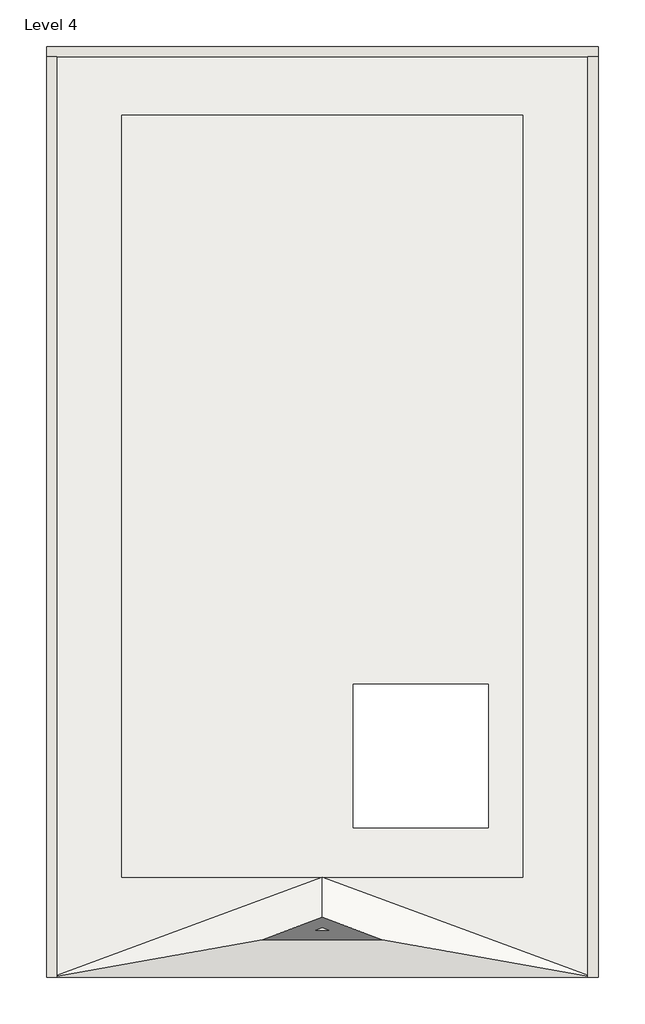
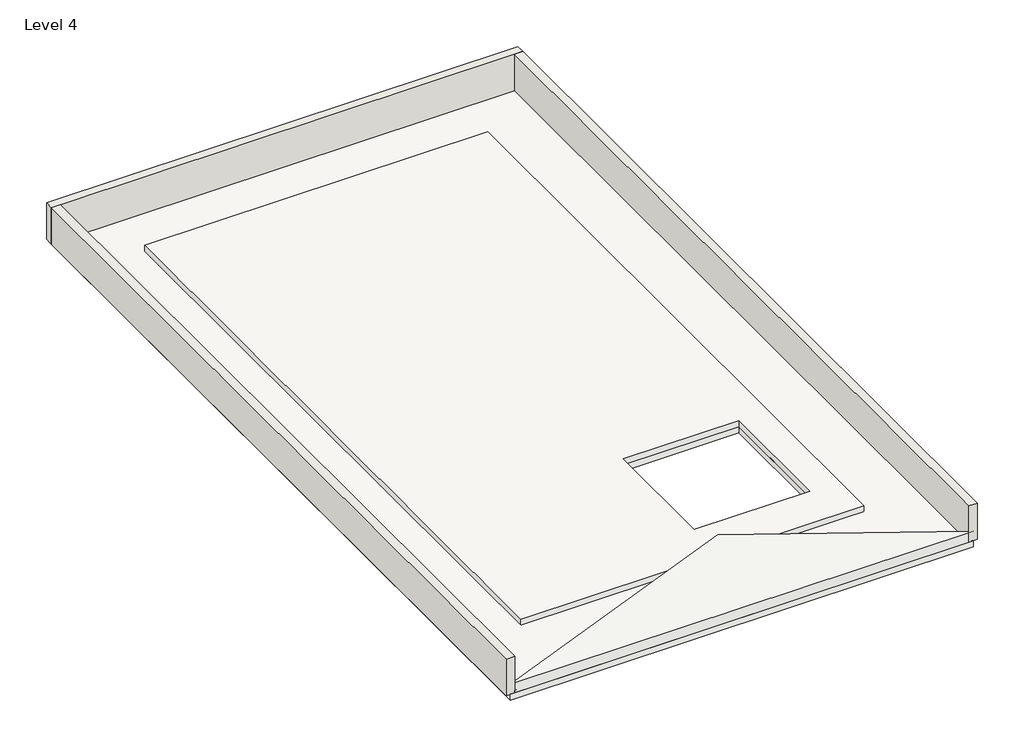
# One storey: 3 walls, 2 roofs, 1 slab.
"""IFC4 building model written with IfcOpenShell, lengths in millimetres."""

from ifc_helpers import new_model, si_unit, frame, origin, place, context, project, spatial, polyline, outline, extrude, faceted_brep, element, save

model = new_model("IFC4")

# Units and contexts
model_context = context("Model", 3, world=origin())
ifc_project = project(units=[si_unit("LENGTHUNIT", "METRE", prefix="MILLI")], contexts=[model_context])

# Site, building, storey
site = spatial("IfcSite", under=ifc_project)
building = spatial("IfcBuilding", under=site)
storey = spatial("IfcBuildingStorey", under=building, Name="Level 4", Elevation=9144.0)

# Roofs
placement = place(None, origin())
element("IfcRoof", 1, ObjectType="Generic - 12\"", at=placement, inside=storey, context=model_context, shape_type="SweptSolid", body=[
    extrude(outline(polyline([(-14949.5126504, -4050.471143), (-14949.5126504, 11392.728857), (-6821.5126504, 11392.728857), (-6821.5126504, -4050.471143), (-14949.5126504, -4050.471143)]), holes=[polyline([(-7518.4, -135.4836), (-10261.6, -135.4836), (-10261.6, -3048.381), (-7518.4, -3048.381), (-7518.4, -135.4836)])]), frame((0.0, 0.0, 9144.0), z_axis=(0.0, 0.0, 1.0), x_axis=(1.0, 0.0, 0.0)), (0.0, 0.0, 1.0), 152.4),
])
element("IfcRoof", 2, ObjectType="Generic - 12\"", at=placement, inside=storey, context=model_context, shape_type="Brep", body=[
    faceted_brep([(-10885.5126504, -5099.110699, 10373.2005551), (-16371.9126504, -6082.471143, 9144.0), (-10885.5126504, -4050.471143, 9144.0), (-5399.1126504, -6082.471143, 9144.0), (-16371.9126504, -6082.471143, 9387.9590334), (-10885.5126504, -5099.110699, 10617.1595885), (-10885.5126504, -4050.471143, 9387.9590334), (-5399.1126504, -6082.471143, 9387.9590334)], [[[0, 1, 2]], [[1, 0, 3]], [[3, 0, 2]], [[4, 5, 6]], [[4, 7, 5]], [[7, 6, 5]], [[3, 7, 4, 1]], [[2, 6, 7, 3]], [[1, 4, 6, 2]]]),
])

# Slab
element("IfcSlab", 3, ObjectType="Generic - 12\"", at=placement, inside=storey, context=model_context, shape_type="SweptSolid", body=[
    extrude(outline(polyline([(-5399.1126504, 12681.3156917), (-5399.1126504, -6082.471143), (-16371.9126504, -6082.471143), (-16371.9126504, 12681.3156917), (-5399.1126504, 12681.3156917)]), holes=[polyline([(-7518.4, -135.4836), (-10261.6, -135.4836), (-10261.6, -3048.381), (-7518.4, -3048.381), (-7518.4, -135.4836)])]), frame((0.0, 0.0, 8991.6), z_axis=(0.0, 0.0, 1.0), x_axis=(1.0, 0.0, 0.0)), (0.0, 0.0, 1.0), 152.4),
])

# Walls
element("IfcWall", 4, ObjectType="Generic - 4.5\" p", at=placement, inside=storey, context=model_context, shape_type="Brep", body=[
    faceted_brep([(-16473.5126504, 12579.7156917, 9144.0), (-16270.3126504, 12579.7156917, 9144.0), (-5500.7126504, 12579.7156917, 9144.0), (-5297.5126504, 12579.7156917, 9144.0), (-5297.5126504, 12579.7156917, 10058.4), (-5500.7126504, 12579.7156917, 10058.4), (-16270.3126504, 12579.7156917, 10058.4), (-16473.5126504, 12579.7156917, 10058.4), (-16473.5126504, 12782.9156917, 9144.0), (-16473.5126504, 12782.9156917, 10058.4), (-5297.5126504, 12782.9156917, 10058.4), (-5297.5126504, 12782.9156917, 9144.0)], [[[0, 1, 2, 3, 4, 5, 6, 7]], [[8, 9, 10, 11]], [[3, 2, 1, 0, 8, 11]], [[7, 6, 5, 4, 10, 9]], [[4, 3, 11, 10]], [[0, 7, 9, 8]]]),
])
element("IfcWall", 5, ObjectType="Generic - 4.5\" p", at=placement, inside=storey, context=model_context, shape_type="SweptSolid", body=[
    extrude(outline(polyline([(-5500.7126504, -6082.471143), (-5500.7126504, 12579.7156917), (-5297.5126504, 12579.7156917), (-5297.5126504, -6082.471143), (-5500.7126504, -6082.471143)])), frame((0.0, 0.0, 9144.0), z_axis=(0.0, 0.0, 1.0), x_axis=(1.0, 0.0, 0.0)), (0.0, 0.0, 1.0), 914.4),
])
element("IfcWall", 6, ObjectType="Generic - 4.5\" p", at=placement, inside=storey, context=model_context, shape_type="SweptSolid", body=[
    extrude(outline(polyline([(-16473.5126504, -6082.471143), (-16473.5126504, 12579.7156917), (-16270.3126504, 12579.7156917), (-16270.3126504, -6082.471143), (-16473.5126504, -6082.471143)])), frame((0.0, 0.0, 9144.0), z_axis=(0.0, 0.0, 1.0), x_axis=(1.0, 0.0, 0.0)), (0.0, 0.0, 1.0), 914.4),
])

save(model, "model.ifc")

# Revit data of these elements
# Type "Generic - 12\""
#   Assembly Code = "B1020"
#   Layers, outside or top first: 0' - 6" no material (function 1)
# Type "Generic - 12\""
#   Assembly Code = "B1010"
#   Function = 0
#   Layers, outside or top first: 0' - 6" no material (function 1)
# Type "Generic - 4.5\" p"
#   Assembly Code = "B2010"
#   Layers, outside or top first: 0' - 8" "Brick, Common" (function 1)
# Element 1 (IfcRoof, "Generic - 12\"")
#   built-in parameter 1001705 = 30.5 (stored number, unit not read)
#   built-in parameter 1001710 = 33615
#   Phase Created = New Construction
#   Materials on its faces: "Default Roof", "Carpet (1)"
# Element 2 (IfcRoof, "Generic - 12\"")
#   built-in parameter 1001705 = 34.8332 (stored number, unit not read)
#   built-in parameter 1001710 = 33615
#   Phase Created = New Construction
#   Materials on its faces: "Default Roof", "Carpet (1)"
# Element 3 (IfcSlab, "Generic - 12\"")
#   Height Offset From Level = 0' - 0"
#   Phase Created = New Construction
#   Materials on its faces: "Default Floor"
# Elements 4, 5, 6 (IfcWall, "Generic - 4.5\" p")
#   Top Offset = 0' - 0"
#   Base Offset = 0' - 0"
#   Unconnected Height = 3' - 0"
#   wall height = 3' - 0"
#   Phase Created = New Construction
#   Base Constraint = Level 4
#   Materials on its faces: "Brick, Common"
# Materials
#   "Brick, Common": class "Masonry", colour RGB 128 0 128, transparency 0, Description = "Common brick", Cost = 0
#   "Default Roof": colour RGB 88 101 114, transparency 0, Cost = 0
#   "Carpet (1)": class "Carpet", colour RGB 124 80 67, transparency 0, Description = "Interior finish", Cost = 0
#   "Default Floor": colour RGB 128 128 128, transparency 0, Cost = 0
